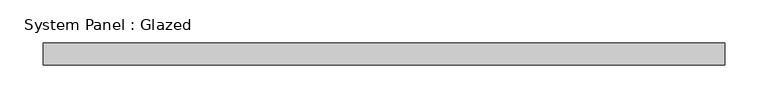
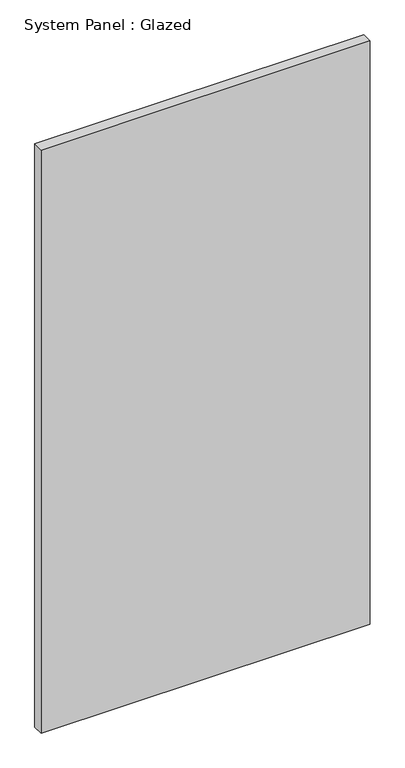
"""IFC4 building model written with IfcOpenShell, lengths in millimetres: plate geometry, System Panel : Glazed."""

from ifc_helpers import new_model, si_unit, origin, origin_with_axes, place, context, project, spatial, polyline, outline, extrude, source, transform, mapped, element, save


def system_panel_glazed_7e5766a3(model_context):
    return source(origin(), model_context, "Body", "SweptSolid", [
        extrude(outline(polyline([(394.9930985, 19.05), (-394.9930985, 19.05), (-394.9930985, 44.45), (394.9930985, 44.45), (394.9930985, 19.05)])), origin_with_axes(), (0.0, 0.0, 1.0), 1478.5835026),
    ])


if __name__ == "__main__":
    model = new_model("IFC4")
    model_context = context("Model", 3, world=origin())
    ifc_project = project(units=[si_unit("LENGTHUNIT", "METRE", prefix="MILLI")], contexts=[model_context])
    site = spatial("IfcSite", under=ifc_project)
    building = spatial("IfcBuilding", under=site)
    placement = place(None, origin())
    system_panel_glazed_shape = system_panel_glazed_7e5766a3(model_context)
    element("IfcPlate", 1, ObjectType="System Panel : Glazed", at=placement, inside=building, context=model_context, shape_type="MappedRepresentation", body=[
        mapped(system_panel_glazed_shape, transform((0.0, 0.0, 0.0), x_axis=(1.0, 0.0, 0.0), y_axis=(0.0, 1.0, 0.0), z_axis=(0.0, 0.0, 1.0))),
    ])
    save(model, "model.ifc")

# Revit data of these elements
# Type "System Panel : Glazed"
#   Construction Type Id = "GSP4R"
#   Analytic Construction = "1/8 in Pilkington single glazing"
#   Visual Light Transmittance = 0.9
#   Solar Heat Gain Coefficient = 0.86
#   Heat Transfer Coefficient (U) = 1.18115 BTU/(h·ft²·°F)
#   Define Thermal Properties by = 1
# Element 1 (IfcPlate, "System Panel : Glazed")
#   Materials on its faces: "Glass"
# Materials
#   "Glass": class "Glass", colour RGB 0 128 192, transparency 0.75, Description = "Soda Lime Glass", Cost = 0
